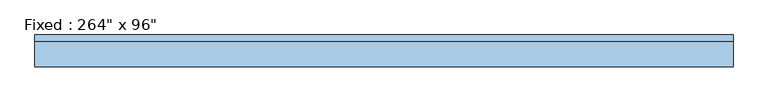
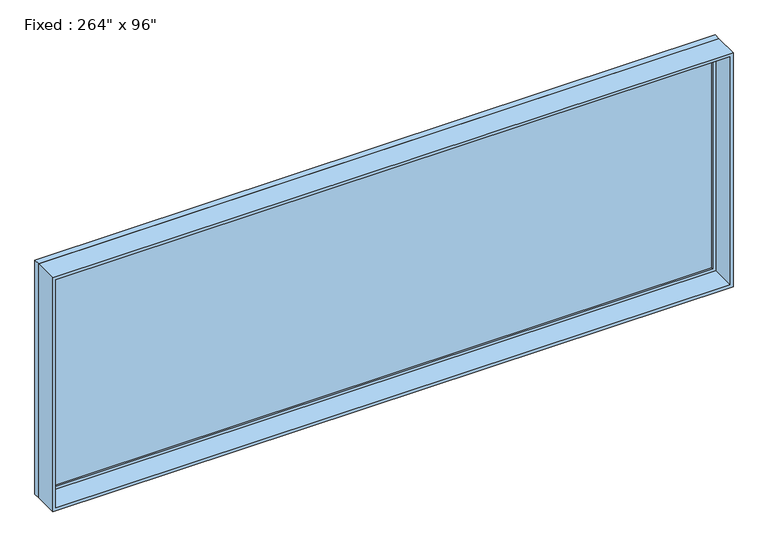
"""IFC4 building model written with IfcOpenShell, lengths in millimetres: window geometry."""

from ifc_helpers import new_model, si_unit, frame, origin, place, context, project, spatial, polyline, outline, extrude, source, transform, mapped, element, save


def window_e4c9328c(model_context):
    return source(origin(), model_context, "Body", "SweptSolid", [
        extrude(outline(polyline([(3251.2, 104.775), (-3327.4, 104.775), (-3327.4, 117.475), (3251.2, 117.475), (3251.2, 104.775)])), frame((0.0, 0.0, 368.3), z_axis=(0.0, 0.0, 1.0), x_axis=(1.0, 0.0, 0.0)), (0.0, 0.0, 1.0), 2311.4),
        extrude(outline(polyline([(2724.15, -3371.85), (323.85, -3371.85), (323.85, 3295.65), (2724.15, 3295.65), (2724.15, -3371.85)]), holes=[polyline([(2679.7, -3327.4), (2679.7, 3251.2), (368.3, 3251.2), (368.3, -3327.4), (2679.7, -3327.4)])]), frame((0.0, 88.9, 0.0), z_axis=(0.0, 1.0, 0.0), x_axis=(0.0, 0.0, 1.0)), (0.0, 0.0, 1.0), 44.45),
        extrude(outline(polyline([(2743.2, -3390.9), (304.8, -3390.9), (304.8, 3314.7), (2743.2, 3314.7), (2743.2, -3390.9)]), holes=[polyline([(2711.45, -3359.15), (2711.45, 3282.95), (336.55, 3282.95), (336.55, -3359.15), (2711.45, -3359.15)])]), frame((0.0, -152.4, 0.0), z_axis=(0.0, 1.0, 0.0), x_axis=(0.0, 0.0, 1.0)), (0.0, 0.0, 1.0), 241.3),
        extrude(outline(polyline([(2743.2, 3314.7), (2743.2, -3390.9), (304.8, -3390.9), (304.8, 3314.7), (2743.2, 3314.7)]), holes=[polyline([(2724.15, 3295.65), (323.85, 3295.65), (323.85, -3371.85), (2724.15, -3371.85), (2724.15, 3295.65)])]), frame((0.0, 88.9, 0.0), z_axis=(0.0, 1.0, 0.0), x_axis=(0.0, 0.0, 1.0)), (0.0, 0.0, 1.0), 63.5),
    ])


if __name__ == "__main__":
    model = new_model("IFC4")
    model_context = context("Model", 3, world=origin())
    ifc_project = project(units=[si_unit("LENGTHUNIT", "METRE", prefix="MILLI")], contexts=[model_context])
    site = spatial("IfcSite", under=ifc_project)
    building = spatial("IfcBuilding", under=site)
    placement = place(None, origin())
    window_shape = window_e4c9328c(model_context)
    element("IfcWindow", 1, ObjectType="Fixed : 264\" x 96\"", at=placement, inside=building, context=model_context, shape_type="MappedRepresentation", body=[
        mapped(window_shape, transform((0.0, 0.0, 0.0), x_axis=(1.0, 0.0, 0.0), y_axis=(0.0, 1.0, 0.0), z_axis=(0.0, 0.0, 1.0))),
    ])
    save(model, "model.ifc")

# Revit data of these elements
# Type "Fixed : 264\" x 96\""
#   Type Mark = "10"
#   Construction Type Id = "GSP4R"
#   Assembly Code = "B2020100"
#   Analytic Construction = "1/8 in Pilkington single glazing"
#   Visual Light Transmittance = 0.9
#   Solar Heat Gain Coefficient = 0.78
#   Heat Transfer Coefficient (U) = 0.6496 BTU/(h·ft²·°F)
#   Height = 8' - 0"
#   Default Sill Height = 1' - 0"
#   Width = 22' - 0"
#   Window Inset = 0' - 0 3/4"
#   Define Thermal Properties by = 1
#   Glass Pane Material = Glass
#   Sash Material = Iron, Ductile
#   Wall Closure = (empty or 0)
# Element 1 (IfcWindow, "Fixed : 264\" x 96\"")
#   Materials on its faces: "Iron, Ductile", "Glass"
# Materials
#   "Glass": class "Glass", colour RGB 0 128 192, transparency 0.75, Description = "Soda Lime Glass", Cost = 0
#   "Iron, Ductile": class "Metal", colour RGB 0 0 0, transparency 0, Description = "Ductile cast iron", Cost = 0
